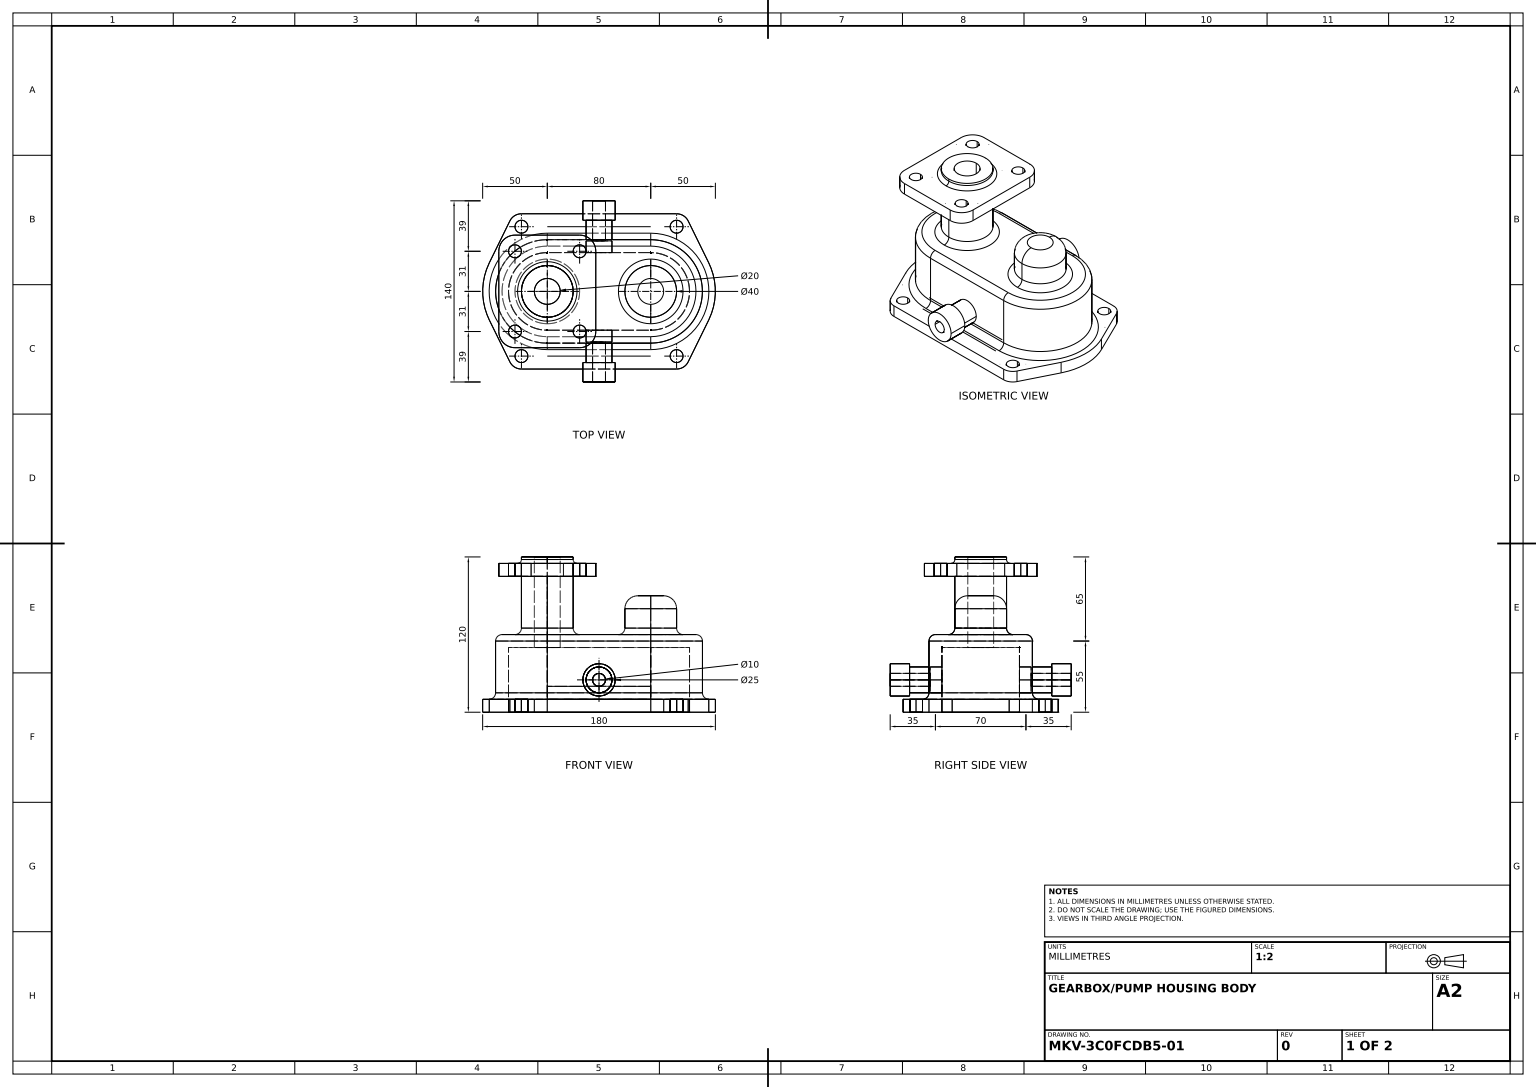
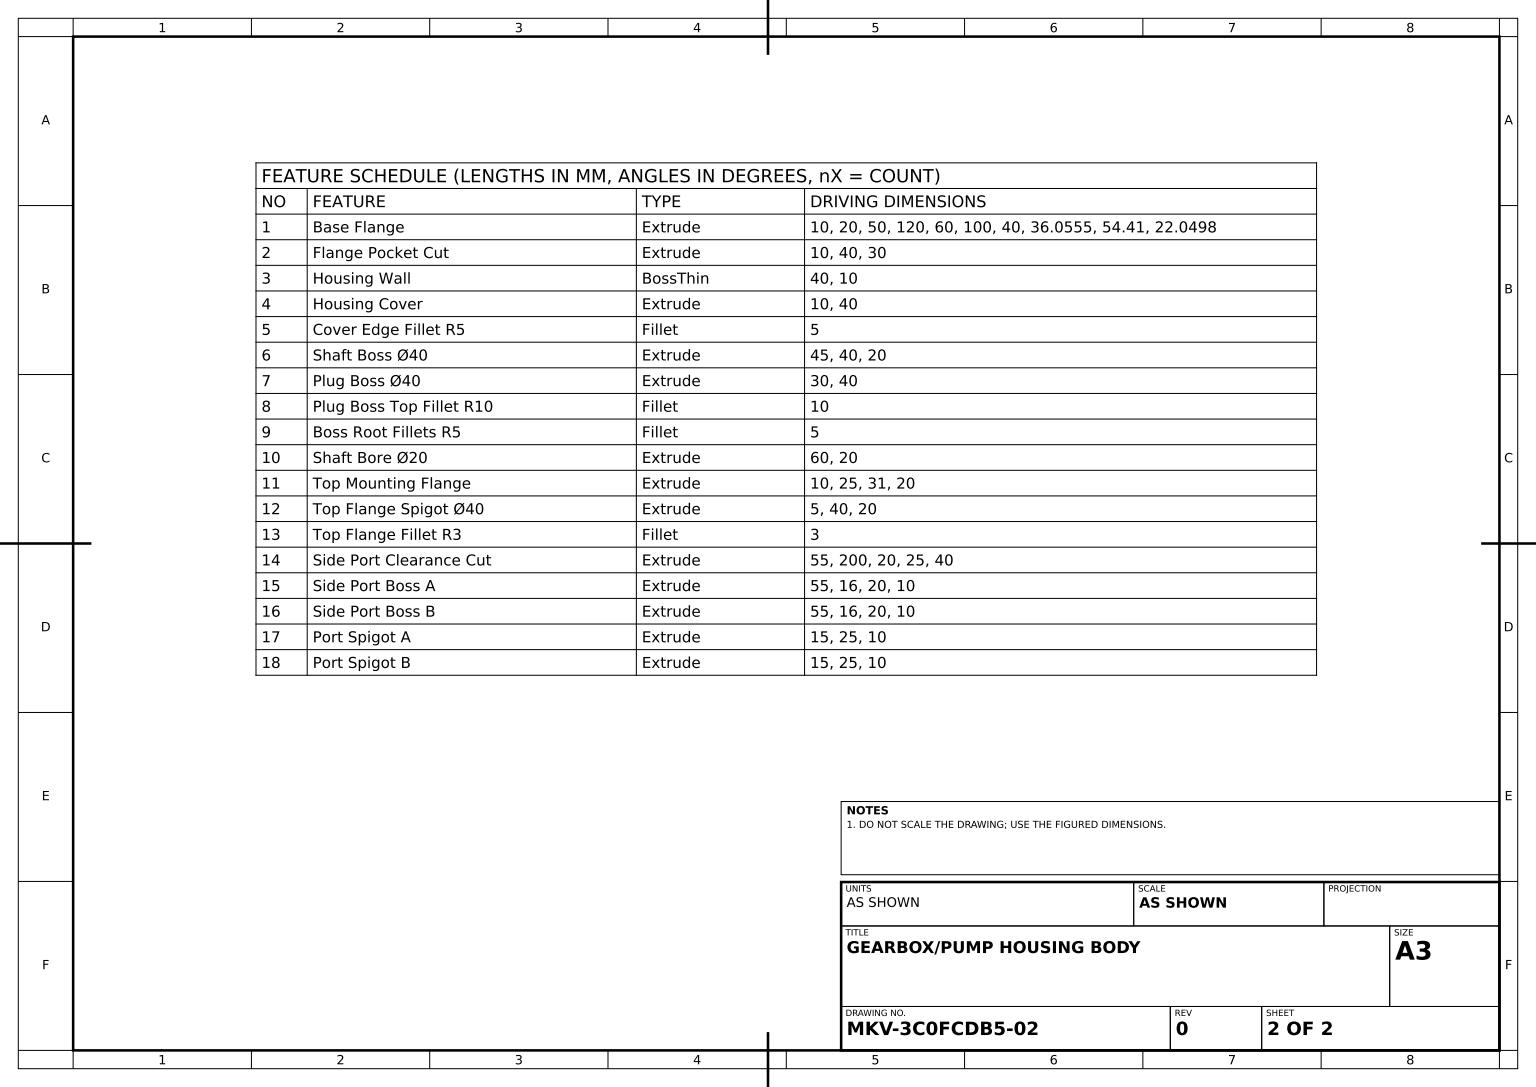
from build123d import *

# Parameters (mm, degrees)
BASE_FLANGE_SKETCH_R           = 5
BASE_FLANGE_DEPTH              = 10
FLANGE_POCKET_CUT_DEPTH        = 10
HOUSING_START                  = 40
HOUSING_WALL_DEPTH             = 40
HOUSING_START_2                = 10
HOUSING_COVER_DEPTH            = 10
COVER_EDGE_FILLET_R5_R         = 5
SHAFT_BOSS_SKETCH_R            = 20
SHAFT_BOSS_SKETCH_R_2          = 10
SHAFT_BOSS_40_DEPTH            = 45
PLUG_BOSS_SKETCH_R             = 20
PLUG_BOSS_40_DEPTH             = 30
PLUG_BOSS_TOP_FILLET_R10_R     = 10
BOSS_ROOT_FILLETS_R5_R         = 5
SHAFT_START                    = -60
SHAFT_BORE_SKETCH_R            = 10
SHAFT_BORE_20_DEPTH            = 60
TOP_MOUNTING_FLANGE_SKETCH_R   = 5
TOP_MOUNTING_FLANGE_SKETCH_R_2 = 10
TOP_MOUNTING_FLANGE_DEPTH      = 10
TOP_FLANGE_SPIGOT_SKETCH_R     = 20
TOP_FLANGE_SPIGOT_SKETCH_R_2   = 10
TOP_FLANGE_SPIGOT_40_DEPTH     = 5
TOP_FLANGE_FILLET_R3_R         = 3
SIDE_PORT_CUT_SKETCH_R         = 10
SIDE_PORT_CLEARANCE_CUT_DEPTH  = 200
SIDE_PORT_BOSS_A_SKETCH_R      = 10
SIDE_PORT_BOSS_A_SKETCH_R_2    = 5
SIDE_PORT_BOSS_A_DEPTH         = 16
SIDE_START                     = 16
SIDE_PORT_BOSS_B_SKETCH_R      = 10
SIDE_PORT_BOSS_B_SKETCH_R_2    = 5
SIDE_PORT_BOSS_B_DEPTH         = 16
PORT_START                     = 15
PORT_SPIGOT_A_SKETCH_R         = 12.5
PORT_SPIGOT_A_SKETCH_R_2       = 5
PORT_SPIGOT_A_DEPTH            = 15
PORT_SPIGOT_B_SKETCH_R         = 12.5
PORT_SPIGOT_B_SKETCH_R_2       = 5
PORT_SPIGOT_B_DEPTH            = 15


with BuildPart() as part:
    # Base Flange Sketch → Base Flange (new body)
    with BuildSketch(Plane(origin=(0, 0, 0), x_dir=(1, 0, 0), z_dir=(0, 1, 0))):
        with BuildLine():
            Line((-60, 60), (60, 60))
            ThreePointArc((60, 60), (65.286792677, 58.488216726), (68.975088406, 54.409964638))
            Line((68.975088406, 54.409964638), (84.87544203, 22.049823188))
            ThreePointArc((84.87544203, 22.049823188), (90, 0), (84.87544203, -22.049823188))
            Line((84.87544203, -22.049823188), (68.975088406, -54.409964638))
            ThreePointArc((68.975088406, -54.409964638), (65.286792677, -58.488216726), (60, -60))
            Line((60, -60), (-60, -60))
            ThreePointArc((-60, -60), (-65.286792677, -58.488216726), (-68.975088406, -54.409964638))
            Line((-68.975088406, -54.409964638), (-84.87544203, -22.049823188))
            ThreePointArc((-84.87544203, -22.049823188), (-90, 0), (-84.87544203, 22.049823188))
            Line((-84.87544203, 22.049823188), (-68.975088406, 54.409964638))
            ThreePointArc((-68.975088406, 54.409964638), (-65.286792677, 58.488216726), (-60, 60))
        make_face()
        with Locations(Location((-60, 50, 0), (0, 0, 270))):
            Circle(BASE_FLANGE_SKETCH_R, mode=Mode.SUBTRACT)
        with Locations(Location((-60, -50, 0), (0, 0, 270))):
            Circle(BASE_FLANGE_SKETCH_R, mode=Mode.SUBTRACT)
        with Locations(Location((60, 50, 0), (0, 0, 270))):
            Circle(BASE_FLANGE_SKETCH_R, mode=Mode.SUBTRACT)
        with Locations(Location((60, -50, 0), (0, 0, 270))):
            Circle(BASE_FLANGE_SKETCH_R, mode=Mode.SUBTRACT)
    extrude(amount=BASE_FLANGE_DEPTH)

    # Flange Pocket Sketch → Flange Pocket Cut (cut)
    with BuildSketch(Plane(origin=(0, 10, 0), x_dir=(1, 0, 0), z_dir=(0, 1, 0))):
        with BuildLine():
            Line((-40, 30), (40, 30))
            ThreePointArc((40, 30), (70, 0), (40, -30))
            Line((40, -30), (-40, -30))
            ThreePointArc((-40, -30), (-70, 0), (-40, 30))
        make_face()
    extrude(amount=-FLANGE_POCKET_CUT_DEPTH, mode=Mode.SUBTRACT)

    # Housing Wall Sketch → Housing Wall (add)
    with BuildSketch(Plane(origin=(0, 10, 0), x_dir=(1, 0, 0), z_dir=(0, 1, 0)).offset(HOUSING_START)):
        with BuildLine():
            Line((40, -40), (-40, -40))
            ThreePointArc((-40, -40), (-80, 0), (-40, 40))
            Line((-40, 40), (40, 40))
            ThreePointArc((40, 40), (80, 0), (40, -40))
        make_face()
        with BuildLine():
            Line((40, -30), (-40, -30))
            ThreePointArc((-40, -30), (-70, 0), (-40, 30))
            Line((-40, 30), (40, 30))
            ThreePointArc((40, 30), (70, 0), (40, -30))
        make_face(mode=Mode.SUBTRACT)
    extrude(amount=-HOUSING_WALL_DEPTH)

    # Housing Cover Sketch → Housing Cover (add)
    with BuildSketch(Plane(origin=(0, 50, 0), x_dir=(1, 0, 0), z_dir=(0, 1, 0)).offset(HOUSING_START_2)):
        with BuildLine():
            Line((-40, 40), (40, 40))
            ThreePointArc((40, 40), (80, 0), (40, -40))
            Line((40, -40), (-40, -40))
            ThreePointArc((-40, -40), (-80, 0), (-40, 40))
        make_face()
    extrude(amount=-HOUSING_COVER_DEPTH)

    # Cover Edge Fillet R5
    cover_edge_fillet_r5_edges = [part.edges().sort_by_distance(p)[0] for p in [
        (-80, 10, 0),
        (0, 10, 40),
        (80, 10, 0),
        (0, 10, -40),
        (-80, 60, 0),
        (0, 60, 40),
        (80, 60, 0),
        (0, 60, -40),
    ]]
    fillet(cover_edge_fillet_r5_edges, radius=COVER_EDGE_FILLET_R5_R)

    # Shaft Boss Sketch → Shaft Boss Ø40 (add)
    with BuildSketch(Plane(origin=(0, 60, 0), x_dir=(1, 0, 0), z_dir=(0, 1, 0))):
        with Locations(Location((-40, 0, 0), (0, 0, 90))):
            Circle(SHAFT_BOSS_SKETCH_R)
        with Locations(Location((-40, 0, 0), (0, 0, 90))):
            Circle(SHAFT_BOSS_SKETCH_R_2, mode=Mode.SUBTRACT)
    extrude(amount=SHAFT_BOSS_40_DEPTH)

    # Plug Boss Sketch → Plug Boss Ø40 (add)
    with BuildSketch(Plane(origin=(0, 60, 0), x_dir=(1, 0, 0), z_dir=(0, 1, 0))):
        with Locations(Location((40, 0, 0), (0, 0, 270))):
            Circle(PLUG_BOSS_SKETCH_R)
    extrude(amount=PLUG_BOSS_40_DEPTH)

    # Plug Boss Top Fillet R10
    plug_boss_top_fillet_r10_edges = [part.edges().sort_by_distance(p)[0] for p in [
        (40, 90, -20),
    ]]
    fillet(plug_boss_top_fillet_r10_edges, radius=PLUG_BOSS_TOP_FILLET_R10_R)

    # Boss Root Fillets R5
    boss_root_fillets_r5_edges = [part.edges().sort_by_distance(p)[0] for p in [
        (-40, 60, 20),
        (40, 60, -20),
    ]]
    fillet(boss_root_fillets_r5_edges, radius=BOSS_ROOT_FILLETS_R5_R)

    # Shaft Bore Sketch → Shaft Bore Ø20 (cut)
    with BuildSketch(Plane(origin=(0, 105, 0), x_dir=(1, 0, 0), z_dir=(0, 1, 0)).offset(SHAFT_START)):
        with Locations(Location((-40, 0, 0), (0, 0, 90))):
            Circle(SHAFT_BORE_SKETCH_R)
    extrude(amount=SHAFT_BORE_20_DEPTH, mode=Mode.SUBTRACT)

    # Top Mounting Flange Sketch → Top Mounting Flange (add)
    with BuildSketch(Plane(origin=(0, 105, 0), x_dir=(1, 0, 0), z_dir=(0, 1, 0))):
        with BuildLine():
            Line((-65, 43.5), (-15, 43.5))
            ThreePointArc((-15, 43.5), (-6.161165235, 39.838834765), (-2.5, 31))
            Line((-2.5, 31), (-2.5, -31))
            ThreePointArc((-2.5, -31), (-6.161165235, -39.838834765), (-15, -43.5))
            Line((-15, -43.5), (-65, -43.5))
            ThreePointArc((-65, -43.5), (-73.838834765, -39.838834765), (-77.5, -31))
            Line((-77.5, -31), (-77.5, 31))
            ThreePointArc((-77.5, 31), (-73.838834765, 39.838834765), (-65, 43.5))
        make_face()
        with Locations(Location((-65, 31, 0), (0, 0, 270))):
            Circle(TOP_MOUNTING_FLANGE_SKETCH_R, mode=Mode.SUBTRACT)
        with Locations(Location((-15, 31, 0), (0, 0, 270))):
            Circle(TOP_MOUNTING_FLANGE_SKETCH_R, mode=Mode.SUBTRACT)
        with Locations(Location((-65, -31, 0), (0, 0, 270))):
            Circle(TOP_MOUNTING_FLANGE_SKETCH_R, mode=Mode.SUBTRACT)
        with Locations(Location((-15, -31, 0), (0, 0, 270))):
            Circle(TOP_MOUNTING_FLANGE_SKETCH_R, mode=Mode.SUBTRACT)
        with Locations(Location((-40, 0, 0), (0, 0, 90))):
            Circle(TOP_MOUNTING_FLANGE_SKETCH_R_2, mode=Mode.SUBTRACT)
    extrude(amount=TOP_MOUNTING_FLANGE_DEPTH)

    # Top Flange Spigot Sketch → Top Flange Spigot Ø40 (add)
    with BuildSketch(Plane(origin=(0, 115, 0), x_dir=(1, 0, 0), z_dir=(0, 1, 0))):
        with Locations(Location((-40, 0, 0), (0, 0, 90))):
            Circle(TOP_FLANGE_SPIGOT_SKETCH_R)
        with Locations(Location((-40, 0, 0), (0, 0, 90))):
            Circle(TOP_FLANGE_SPIGOT_SKETCH_R_2, mode=Mode.SUBTRACT)
    extrude(amount=TOP_FLANGE_SPIGOT_40_DEPTH)

    # Top Flange Fillet R3
    top_flange_fillet_r3_edges = [part.edges().sort_by_distance(p)[0] for p in [
        (-40, 115, 20),
    ]]
    fillet(top_flange_fillet_r3_edges, radius=TOP_FLANGE_FILLET_R3_R)

    # Side Port Cut Sketch → Side Port Clearance Cut (cut)
    with BuildSketch(Plane.XY.offset(55)):
        with Locations(Location((0, 25, 0), (0, 0, 270))):
            Circle(SIDE_PORT_CUT_SKETCH_R)
    extrude(amount=-SIDE_PORT_CLEARANCE_CUT_DEPTH, mode=Mode.SUBTRACT)

    # Side Port Boss A Sketch → Side Port Boss A (add)
    with BuildSketch(Plane.XY.offset(55)):
        with Locations((0, 25)):
            Circle(SIDE_PORT_BOSS_A_SKETCH_R)
        with Locations((0, 25)):
            Circle(SIDE_PORT_BOSS_A_SKETCH_R_2, mode=Mode.SUBTRACT)
    extrude(amount=-SIDE_PORT_BOSS_A_DEPTH)

    # Side Port Boss B Sketch → Side Port Boss B (add)
    with BuildSketch(Plane.XY.offset(-55).offset(SIDE_START)):
        with Locations((0, 25)):
            Circle(SIDE_PORT_BOSS_B_SKETCH_R)
        with Locations((0, 25)):
            Circle(SIDE_PORT_BOSS_B_SKETCH_R_2, mode=Mode.SUBTRACT)
    extrude(amount=-SIDE_PORT_BOSS_B_DEPTH)

    # Port Spigot A Sketch → Port Spigot A (add)
    with BuildSketch(Plane.XY.offset(55).offset(PORT_START)):
        with Locations((0, 25)):
            Circle(PORT_SPIGOT_A_SKETCH_R)
        with Locations((0, 25)):
            Circle(PORT_SPIGOT_A_SKETCH_R_2, mode=Mode.SUBTRACT)
    extrude(amount=-PORT_SPIGOT_A_DEPTH)

    # Port Spigot B Sketch → Port Spigot B (add)
    with BuildSketch(Plane(origin=(0, 0, -55), x_dir=(-1, 0, 0), z_dir=(0, 0, -1))):
        with Locations(Location((0, 25, 0), (0, 0, 180))):
            Circle(PORT_SPIGOT_B_SKETCH_R)
        with Locations(Location((0, 25, 0), (0, 0, 180))):
            Circle(PORT_SPIGOT_B_SKETCH_R_2, mode=Mode.SUBTRACT)
    extrude(amount=PORT_SPIGOT_B_DEPTH)


solid = part.part
